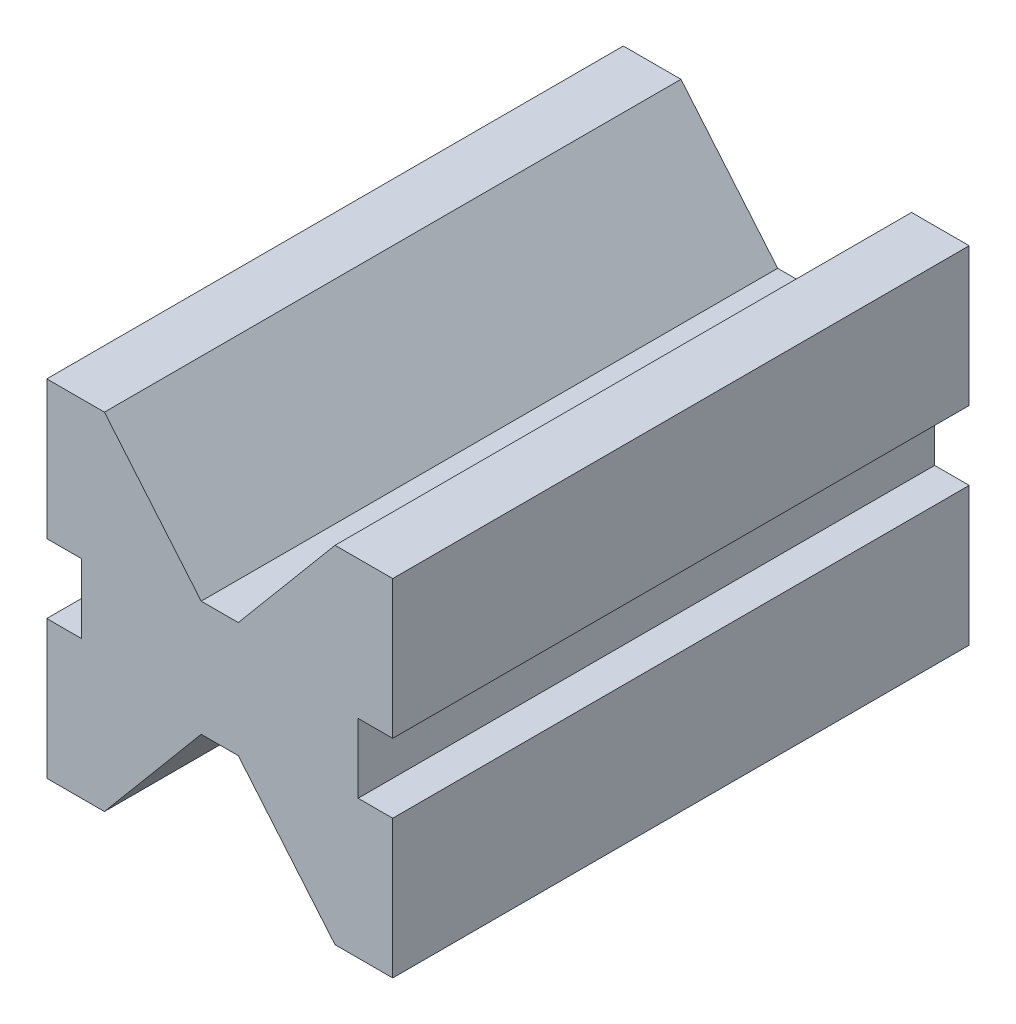
ISO-10303-21;
HEADER;
FILE_DESCRIPTION(('STEP AP214'),'2;1');
FILE_NAME('part.step','',(''),(''),'','','');
FILE_SCHEMA(('AUTOMOTIVE_DESIGN { 1 0 10303 214 1 1 1 1 }'));
ENDSEC;
DATA;
#1=APPLICATION_CONTEXT('core data for automotive mechanical design processes');
#2=APPLICATION_PROTOCOL_DEFINITION('international standard','automotive_design',2000,#1);
#3=PRODUCT_CONTEXT('',#1,'mechanical');
#4=PRODUCT('Part','Part','',(#3));
#5=PRODUCT_RELATED_PRODUCT_CATEGORY('part','',(#4));
#6=PRODUCT_DEFINITION_FORMATION('','',#4);
#7=PRODUCT_DEFINITION_CONTEXT('part definition',#1,'design');
#8=PRODUCT_DEFINITION('design','',#6,#7);
#9=PRODUCT_DEFINITION_SHAPE('','',#8);
#10=(LENGTH_UNIT() NAMED_UNIT(*) SI_UNIT(.MILLI.,.METRE.));
#11=(NAMED_UNIT(*) PLANE_ANGLE_UNIT() SI_UNIT($,.RADIAN.));
#12=(NAMED_UNIT(*) SI_UNIT($,.STERADIAN.) SOLID_ANGLE_UNIT());
#13=UNCERTAINTY_MEASURE_WITH_UNIT(LENGTH_MEASURE(1.E-05),#10,'distance_accuracy_value','');
#14=(GEOMETRIC_REPRESENTATION_CONTEXT(3) GLOBAL_UNCERTAINTY_ASSIGNED_CONTEXT((#13)) GLOBAL_UNIT_ASSIGNED_CONTEXT((#10,
#11,#12)) REPRESENTATION_CONTEXT('',''));
#15=CARTESIAN_POINT('',(0.,0.,0.));
#16=DIRECTION('',(0.,0.,1.));
#17=DIRECTION('',(1.,0.,0.));
#18=AXIS2_PLACEMENT_3D('',#15,#16,#17);
#19=CARTESIAN_POINT('',(3.03563451851378,2.54719980487392,-100.));
#20=DIRECTION('',(-0.766044443118979,-0.642787609686538,0.));
#21=DIRECTION('',(0.642787609686538,-0.766044443118979,0.));
#22=AXIS2_PLACEMENT_3D('',#19,#20,#21);
#23=PLANE('',#22);
#24=DIRECTION('',(0.642787609686538,-0.766044443118979,0.));
#25=VECTOR('',#24,1.);
#26=CARTESIAN_POINT('',(3.03563451851378,2.54719980487392,0.));
#27=LINE('',#26,#25);
#28=CARTESIAN_POINT('',(-20.,30.,0.));
#29=VERTEX_POINT('',#28);
#30=CARTESIAN_POINT('',(-3.21800737645446,10.,0.));
#31=VERTEX_POINT('',#30);
#32=EDGE_CURVE('E209',#29,#31,#27,.T.);
#33=ORIENTED_EDGE('',*,*,#32,.T.);
#34=DIRECTION('',(0.,0.,1.));
#35=VECTOR('',#34,1.);
#36=CARTESIAN_POINT('',(-3.21800737645446,10.,-100.));
#37=LINE('',#36,#35);
#38=CARTESIAN_POINT('',(-3.21800737645446,10.,-100.));
#39=VERTEX_POINT('',#38);
#40=EDGE_CURVE('E11',#39,#31,#37,.T.);
#41=ORIENTED_EDGE('',*,*,#40,.F.);
#42=DIRECTION('',(0.642787609686538,-0.766044443118979,0.));
#43=VECTOR('',#42,1.);
#44=CARTESIAN_POINT('',(3.03563451851378,2.54719980487392,-100.));
#45=LINE('',#44,#43);
#46=CARTESIAN_POINT('',(-20.,30.,-100.));
#47=VERTEX_POINT('',#46);
#48=EDGE_CURVE('E257',#47,#39,#45,.T.);
#49=ORIENTED_EDGE('',*,*,#48,.F.);
#50=DIRECTION('',(0.,0.,1.));
#51=VECTOR('',#50,1.);
#52=CARTESIAN_POINT('',(-20.,30.,-100.));
#53=LINE('',#52,#51);
#54=EDGE_CURVE('E42',#47,#29,#53,.T.);
#55=ORIENTED_EDGE('',*,*,#54,.T.);
#56=EDGE_LOOP('',(#33,#41,#49,#55));
#57=FACE_BOUND('',#56,.T.);
#58=ADVANCED_FACE('F41',(#57),#23,.F.);
#59=CARTESIAN_POINT('',(0.,10.,-100.));
#60=DIRECTION('',(0.,-1.,0.));
#61=DIRECTION('',(1.,0.,0.));
#62=AXIS2_PLACEMENT_3D('',#59,#60,#61);
#63=PLANE('',#62);
#64=DIRECTION('',(1.,0.,0.));
#65=VECTOR('',#64,1.);
#66=CARTESIAN_POINT('',(0.,10.,0.));
#67=LINE('',#66,#65);
#68=CARTESIAN_POINT('',(3.21800737645446,10.,0.));
#69=VERTEX_POINT('',#68);
#70=EDGE_CURVE('E126',#31,#69,#67,.T.);
#71=ORIENTED_EDGE('',*,*,#70,.T.);
#72=DIRECTION('',(0.,0.,1.));
#73=VECTOR('',#72,1.);
#74=CARTESIAN_POINT('',(3.21800737645446,10.,-100.));
#75=LINE('',#74,#73);
#76=CARTESIAN_POINT('',(3.21800737645446,10.,-100.));
#77=VERTEX_POINT('',#76);
#78=EDGE_CURVE('E49',#77,#69,#75,.T.);
#79=ORIENTED_EDGE('',*,*,#78,.F.);
#80=DIRECTION('',(1.,0.,0.));
#81=VECTOR('',#80,1.);
#82=CARTESIAN_POINT('',(0.,10.,-100.));
#83=LINE('',#82,#81);
#84=EDGE_CURVE('E59',#39,#77,#83,.T.);
#85=ORIENTED_EDGE('',*,*,#84,.F.);
#86=ORIENTED_EDGE('',*,*,#40,.T.);
#87=EDGE_LOOP('',(#71,#79,#85,#86));
#88=FACE_BOUND('',#87,.T.);
#89=ADVANCED_FACE('F311',(#88),#63,.F.);
#90=CARTESIAN_POINT('',(-3.03563451851378,2.54719980487392,-100.));
#91=DIRECTION('',(-0.766044443118979,0.642787609686538,0.));
#92=DIRECTION('',(-0.642787609686538,-0.766044443118979,0.));
#93=AXIS2_PLACEMENT_3D('',#90,#91,#92);
#94=PLANE('',#93);
#95=DIRECTION('',(-0.642787609686538,-0.766044443118979,0.));
#96=VECTOR('',#95,1.);
#97=CARTESIAN_POINT('',(-3.03563451851378,2.54719980487392,0.));
#98=LINE('',#97,#96);
#99=CARTESIAN_POINT('',(20.,30.,0.));
#100=VERTEX_POINT('',#99);
#101=EDGE_CURVE('E187',#100,#69,#98,.T.);
#102=ORIENTED_EDGE('',*,*,#101,.F.);
#103=DIRECTION('',(0.,0.,1.));
#104=VECTOR('',#103,1.);
#105=CARTESIAN_POINT('',(20.,30.,-100.));
#106=LINE('',#105,#104);
#107=CARTESIAN_POINT('',(20.,30.,-100.));
#108=VERTEX_POINT('',#107);
#109=EDGE_CURVE('E184',#108,#100,#106,.T.);
#110=ORIENTED_EDGE('',*,*,#109,.F.);
#111=DIRECTION('',(-0.642787609686538,-0.766044443118979,0.));
#112=VECTOR('',#111,1.);
#113=CARTESIAN_POINT('',(-3.03563451851378,2.54719980487392,-100.));
#114=LINE('',#113,#112);
#115=EDGE_CURVE('E190',#108,#77,#114,.T.);
#116=ORIENTED_EDGE('',*,*,#115,.T.);
#117=ORIENTED_EDGE('',*,*,#78,.T.);
#118=EDGE_LOOP('',(#102,#110,#116,#117));
#119=FACE_BOUND('',#118,.T.);
#120=ADVANCED_FACE('F186',(#119),#94,.T.);
#121=CARTESIAN_POINT('',(0.,30.,-100.));
#122=DIRECTION('',(0.,1.,0.));
#123=DIRECTION('',(-1.,0.,0.));
#124=AXIS2_PLACEMENT_3D('',#121,#122,#123);
#125=PLANE('',#124);
#126=DIRECTION('',(-1.,0.,0.));
#127=VECTOR('',#126,1.);
#128=CARTESIAN_POINT('',(0.,30.,0.));
#129=LINE('',#128,#127);
#130=CARTESIAN_POINT('',(30.,30.,0.));
#131=VERTEX_POINT('',#130);
#132=EDGE_CURVE('E260',#131,#100,#129,.T.);
#133=ORIENTED_EDGE('',*,*,#132,.F.);
#134=DIRECTION('',(0.,0.,1.));
#135=VECTOR('',#134,1.);
#136=CARTESIAN_POINT('',(30.,30.,-100.));
#137=LINE('',#136,#135);
#138=CARTESIAN_POINT('',(30.,30.,-100.));
#139=VERTEX_POINT('',#138);
#140=EDGE_CURVE('E195',#139,#131,#137,.T.);
#141=ORIENTED_EDGE('',*,*,#140,.F.);
#142=DIRECTION('',(-1.,0.,0.));
#143=VECTOR('',#142,1.);
#144=CARTESIAN_POINT('',(0.,30.,-100.));
#145=LINE('',#144,#143);
#146=EDGE_CURVE('E200',#139,#108,#145,.T.);
#147=ORIENTED_EDGE('',*,*,#146,.T.);
#148=ORIENTED_EDGE('',*,*,#109,.T.);
#149=EDGE_LOOP('',(#133,#141,#147,#148));
#150=FACE_BOUND('',#149,.T.);
#151=ADVANCED_FACE('F205',(#150),#125,.T.);
#152=CARTESIAN_POINT('',(30.,0.,-100.));
#153=DIRECTION('',(1.,0.,0.));
#154=DIRECTION('',(0.,0.,-1.));
#155=AXIS2_PLACEMENT_3D('',#152,#153,#154);
#156=PLANE('',#155);
#157=DIRECTION('',(0.,1.,0.));
#158=VECTOR('',#157,1.);
#159=CARTESIAN_POINT('',(30.,0.,0.));
#160=LINE('',#159,#158);
#161=CARTESIAN_POINT('',(30.,5.99999999999999,0.));
#162=VERTEX_POINT('',#161);
#163=EDGE_CURVE('E255',#162,#131,#160,.T.);
#164=ORIENTED_EDGE('',*,*,#163,.F.);
#165=DIRECTION('',(0.,0.,1.));
#166=VECTOR('',#165,1.);
#167=CARTESIAN_POINT('',(30.,5.99999999999999,-100.));
#168=LINE('',#167,#166);
#169=CARTESIAN_POINT('',(30.,5.99999999999999,-100.));
#170=VERTEX_POINT('',#169);
#171=EDGE_CURVE('E262',#170,#162,#168,.T.);
#172=ORIENTED_EDGE('',*,*,#171,.F.);
#173=DIRECTION('',(0.,1.,0.));
#174=VECTOR('',#173,1.);
#175=CARTESIAN_POINT('',(30.,0.,-100.));
#176=LINE('',#175,#174);
#177=EDGE_CURVE('E201',#170,#139,#176,.T.);
#178=ORIENTED_EDGE('',*,*,#177,.T.);
#179=ORIENTED_EDGE('',*,*,#140,.T.);
#180=EDGE_LOOP('',(#164,#172,#178,#179));
#181=FACE_BOUND('',#180,.T.);
#182=ADVANCED_FACE('F326',(#181),#156,.T.);
#183=CARTESIAN_POINT('',(0.,5.99999999999999,-100.));
#184=DIRECTION('',(0.,1.,0.));
#185=DIRECTION('',(-1.,0.,0.));
#186=AXIS2_PLACEMENT_3D('',#183,#184,#185);
#187=PLANE('',#186);
#188=DIRECTION('',(-1.,0.,0.));
#189=VECTOR('',#188,1.);
#190=CARTESIAN_POINT('',(0.,5.99999999999999,0.));
#191=LINE('',#190,#189);
#192=CARTESIAN_POINT('',(24.,5.99999999999999,0.));
#193=VERTEX_POINT('',#192);
#194=EDGE_CURVE('E252',#162,#193,#191,.T.);
#195=ORIENTED_EDGE('',*,*,#194,.T.);
#196=DIRECTION('',(0.,0.,1.));
#197=VECTOR('',#196,1.);
#198=CARTESIAN_POINT('',(24.,5.99999999999999,-100.));
#199=LINE('',#198,#197);
#200=CARTESIAN_POINT('',(24.,5.99999999999999,-100.));
#201=VERTEX_POINT('',#200);
#202=EDGE_CURVE('E266',#201,#193,#199,.T.);
#203=ORIENTED_EDGE('',*,*,#202,.F.);
#204=DIRECTION('',(-1.,0.,0.));
#205=VECTOR('',#204,1.);
#206=CARTESIAN_POINT('',(0.,5.99999999999999,-100.));
#207=LINE('',#206,#205);
#208=EDGE_CURVE('E202',#170,#201,#207,.T.);
#209=ORIENTED_EDGE('',*,*,#208,.F.);
#210=ORIENTED_EDGE('',*,*,#171,.T.);
#211=EDGE_LOOP('',(#195,#203,#209,#210));
#212=FACE_BOUND('',#211,.T.);
#213=ADVANCED_FACE('F328',(#212),#187,.F.);
#214=CARTESIAN_POINT('',(24.,0.,-100.));
#215=DIRECTION('',(-1.,0.,0.));
#216=DIRECTION('',(0.,0.,1.));
#217=AXIS2_PLACEMENT_3D('',#214,#215,#216);
#218=PLANE('',#217);
#219=DIRECTION('',(0.,-1.,0.));
#220=VECTOR('',#219,1.);
#221=CARTESIAN_POINT('',(24.,0.,0.));
#222=LINE('',#221,#220);
#223=CARTESIAN_POINT('',(24.,-6.00000000000001,0.));
#224=VERTEX_POINT('',#223);
#225=EDGE_CURVE('E248',#193,#224,#222,.T.);
#226=ORIENTED_EDGE('',*,*,#225,.T.);
#227=DIRECTION('',(0.,0.,1.));
#228=VECTOR('',#227,1.);
#229=CARTESIAN_POINT('',(24.,-6.00000000000001,-100.));
#230=LINE('',#229,#228);
#231=CARTESIAN_POINT('',(24.,-6.00000000000001,-100.));
#232=VERTEX_POINT('',#231);
#233=EDGE_CURVE('E267',#232,#224,#230,.T.);
#234=ORIENTED_EDGE('',*,*,#233,.F.);
#235=DIRECTION('',(0.,-1.,0.));
#236=VECTOR('',#235,1.);
#237=CARTESIAN_POINT('',(24.,0.,-100.));
#238=LINE('',#237,#236);
#239=EDGE_CURVE('E423',#201,#232,#238,.T.);
#240=ORIENTED_EDGE('',*,*,#239,.F.);
#241=ORIENTED_EDGE('',*,*,#202,.T.);
#242=EDGE_LOOP('',(#226,#234,#240,#241));
#243=FACE_BOUND('',#242,.T.);
#244=ADVANCED_FACE('F334',(#243),#218,.F.);
#245=CARTESIAN_POINT('',(0.,-6.00000000000001,-100.));
#246=DIRECTION('',(0.,-1.,0.));
#247=DIRECTION('',(0.,0.,-1.));
#248=AXIS2_PLACEMENT_3D('',#245,#246,#247);
#249=PLANE('',#248);
#250=DIRECTION('',(1.,0.,0.));
#251=VECTOR('',#250,1.);
#252=CARTESIAN_POINT('',(0.,-6.00000000000001,0.));
#253=LINE('',#252,#251);
#254=CARTESIAN_POINT('',(30.,-6.00000000000001,0.));
#255=VERTEX_POINT('',#254);
#256=EDGE_CURVE('E249',#224,#255,#253,.T.);
#257=ORIENTED_EDGE('',*,*,#256,.T.);
#258=DIRECTION('',(0.,0.,1.));
#259=VECTOR('',#258,1.);
#260=CARTESIAN_POINT('',(30.,-6.00000000000001,-100.));
#261=LINE('',#260,#259);
#262=CARTESIAN_POINT('',(30.,-6.00000000000001,-100.));
#263=VERTEX_POINT('',#262);
#264=EDGE_CURVE('E275',#263,#255,#261,.T.);
#265=ORIENTED_EDGE('',*,*,#264,.F.);
#266=DIRECTION('',(1.,0.,0.));
#267=VECTOR('',#266,1.);
#268=CARTESIAN_POINT('',(0.,-6.00000000000001,-100.));
#269=LINE('',#268,#267);
#270=EDGE_CURVE('E420',#232,#263,#269,.T.);
#271=ORIENTED_EDGE('',*,*,#270,.F.);
#272=ORIENTED_EDGE('',*,*,#233,.T.);
#273=EDGE_LOOP('',(#257,#265,#271,#272));
#274=FACE_BOUND('',#273,.T.);
#275=ADVANCED_FACE('F340',(#274),#249,.F.);
#276=CARTESIAN_POINT('',(30.,0.,-100.));
#277=DIRECTION('',(1.,0.,0.));
#278=DIRECTION('',(0.,0.,-1.));
#279=AXIS2_PLACEMENT_3D('',#276,#277,#278);
#280=PLANE('',#279);
#281=DIRECTION('',(0.,1.,0.));
#282=VECTOR('',#281,1.);
#283=CARTESIAN_POINT('',(30.,0.,0.));
#284=LINE('',#283,#282);
#285=CARTESIAN_POINT('',(30.,-30.,0.));
#286=VERTEX_POINT('',#285);
#287=EDGE_CURVE('E243',#286,#255,#284,.T.);
#288=ORIENTED_EDGE('',*,*,#287,.F.);
#289=DIRECTION('',(0.,0.,1.));
#290=VECTOR('',#289,1.);
#291=CARTESIAN_POINT('',(30.,-30.,-100.));
#292=LINE('',#291,#290);
#293=CARTESIAN_POINT('',(30.,-30.,-100.));
#294=VERTEX_POINT('',#293);
#295=EDGE_CURVE('E273',#294,#286,#292,.T.);
#296=ORIENTED_EDGE('',*,*,#295,.F.);
#297=DIRECTION('',(0.,1.,0.));
#298=VECTOR('',#297,1.);
#299=CARTESIAN_POINT('',(30.,0.,-100.));
#300=LINE('',#299,#298);
#301=EDGE_CURVE('E418',#294,#263,#300,.T.);
#302=ORIENTED_EDGE('',*,*,#301,.T.);
#303=ORIENTED_EDGE('',*,*,#264,.T.);
#304=EDGE_LOOP('',(#288,#296,#302,#303));
#305=FACE_BOUND('',#304,.T.);
#306=ADVANCED_FACE('F342',(#305),#280,.T.);
#307=CARTESIAN_POINT('',(0.,-30.,-100.));
#308=DIRECTION('',(0.,-1.,0.));
#309=DIRECTION('',(0.,0.,-1.));
#310=AXIS2_PLACEMENT_3D('',#307,#308,#309);
#311=PLANE('',#310);
#312=DIRECTION('',(1.,0.,0.));
#313=VECTOR('',#312,1.);
#314=CARTESIAN_POINT('',(0.,-30.,0.));
#315=LINE('',#314,#313);
#316=CARTESIAN_POINT('',(20.,-30.,0.));
#317=VERTEX_POINT('',#316);
#318=EDGE_CURVE('E241',#317,#286,#315,.T.);
#319=ORIENTED_EDGE('',*,*,#318,.F.);
#320=DIRECTION('',(0.,0.,1.));
#321=VECTOR('',#320,1.);
#322=CARTESIAN_POINT('',(20.,-30.,-100.));
#323=LINE('',#322,#321);
#324=CARTESIAN_POINT('',(20.,-30.,-100.));
#325=VERTEX_POINT('',#324);
#326=EDGE_CURVE('E277',#325,#317,#323,.T.);
#327=ORIENTED_EDGE('',*,*,#326,.F.);
#328=DIRECTION('',(1.,0.,0.));
#329=VECTOR('',#328,1.);
#330=CARTESIAN_POINT('',(0.,-30.,-100.));
#331=LINE('',#330,#329);
#332=EDGE_CURVE('E415',#325,#294,#331,.T.);
#333=ORIENTED_EDGE('',*,*,#332,.T.);
#334=ORIENTED_EDGE('',*,*,#295,.T.);
#335=EDGE_LOOP('',(#319,#327,#333,#334));
#336=FACE_BOUND('',#335,.T.);
#337=ADVANCED_FACE('F343',(#336),#311,.T.);
#338=CARTESIAN_POINT('',(-3.03563451851378,-2.54719980487392,-100.));
#339=DIRECTION('',(0.766044443118979,0.642787609686538,0.));
#340=DIRECTION('',(-0.642787609686538,0.766044443118979,0.));
#341=AXIS2_PLACEMENT_3D('',#338,#339,#340);
#342=PLANE('',#341);
#343=DIRECTION('',(-0.642787609686538,0.766044443118979,0.));
#344=VECTOR('',#343,1.);
#345=CARTESIAN_POINT('',(-3.03563451851378,-2.54719980487392,0.));
#346=LINE('',#345,#344);
#347=CARTESIAN_POINT('',(3.21800737645446,-10.,0.));
#348=VERTEX_POINT('',#347);
#349=EDGE_CURVE('E239',#317,#348,#346,.T.);
#350=ORIENTED_EDGE('',*,*,#349,.T.);
#351=DIRECTION('',(0.,0.,1.));
#352=VECTOR('',#351,1.);
#353=CARTESIAN_POINT('',(3.21800737645446,-10.,-100.));
#354=LINE('',#353,#352);
#355=CARTESIAN_POINT('',(3.21800737645446,-10.,-100.));
#356=VERTEX_POINT('',#355);
#357=EDGE_CURVE('E279',#356,#348,#354,.T.);
#358=ORIENTED_EDGE('',*,*,#357,.F.);
#359=DIRECTION('',(-0.642787609686538,0.766044443118979,0.));
#360=VECTOR('',#359,1.);
#361=CARTESIAN_POINT('',(-3.03563451851378,-2.54719980487392,-100.));
#362=LINE('',#361,#360);
#363=EDGE_CURVE('E412',#325,#356,#362,.T.);
#364=ORIENTED_EDGE('',*,*,#363,.F.);
#365=ORIENTED_EDGE('',*,*,#326,.T.);
#366=EDGE_LOOP('',(#350,#358,#364,#365));
#367=FACE_BOUND('',#366,.T.);
#368=ADVANCED_FACE('F349',(#367),#342,.F.);
#369=CARTESIAN_POINT('',(0.,-10.,-100.));
#370=DIRECTION('',(0.,1.,0.));
#371=DIRECTION('',(-1.,0.,0.));
#372=AXIS2_PLACEMENT_3D('',#369,#370,#371);
#373=PLANE('',#372);
#374=DIRECTION('',(-1.,0.,0.));
#375=VECTOR('',#374,1.);
#376=CARTESIAN_POINT('',(0.,-10.,0.));
#377=LINE('',#376,#375);
#378=CARTESIAN_POINT('',(-3.21800737645446,-10.,0.));
#379=VERTEX_POINT('',#378);
#380=EDGE_CURVE('E237',#348,#379,#377,.T.);
#381=ORIENTED_EDGE('',*,*,#380,.T.);
#382=DIRECTION('',(0.,0.,1.));
#383=VECTOR('',#382,1.);
#384=CARTESIAN_POINT('',(-3.21800737645446,-10.,-100.));
#385=LINE('',#384,#383);
#386=CARTESIAN_POINT('',(-3.21800737645446,-10.,-100.));
#387=VERTEX_POINT('',#386);
#388=EDGE_CURVE('E281',#387,#379,#385,.T.);
#389=ORIENTED_EDGE('',*,*,#388,.F.);
#390=DIRECTION('',(-1.,0.,0.));
#391=VECTOR('',#390,1.);
#392=CARTESIAN_POINT('',(0.,-10.,-100.));
#393=LINE('',#392,#391);
#394=EDGE_CURVE('E408',#356,#387,#393,.T.);
#395=ORIENTED_EDGE('',*,*,#394,.F.);
#396=ORIENTED_EDGE('',*,*,#357,.T.);
#397=EDGE_LOOP('',(#381,#389,#395,#396));
#398=FACE_BOUND('',#397,.T.);
#399=ADVANCED_FACE('F352',(#398),#373,.F.);
#400=CARTESIAN_POINT('',(3.03563451851378,-2.54719980487392,-100.));
#401=DIRECTION('',(0.766044443118979,-0.642787609686538,0.));
#402=DIRECTION('',(0.642787609686538,0.766044443118979,0.));
#403=AXIS2_PLACEMENT_3D('',#400,#401,#402);
#404=PLANE('',#403);
#405=DIRECTION('',(0.642787609686538,0.766044443118979,0.));
#406=VECTOR('',#405,1.);
#407=CARTESIAN_POINT('',(3.03563451851378,-2.54719980487392,0.));
#408=LINE('',#407,#406);
#409=CARTESIAN_POINT('',(-20.,-30.,0.));
#410=VERTEX_POINT('',#409);
#411=EDGE_CURVE('E235',#410,#379,#408,.T.);
#412=ORIENTED_EDGE('',*,*,#411,.F.);
#413=DIRECTION('',(0.,0.,1.));
#414=VECTOR('',#413,1.);
#415=CARTESIAN_POINT('',(-20.,-30.,-100.));
#416=LINE('',#415,#414);
#417=CARTESIAN_POINT('',(-20.,-30.,-100.));
#418=VERTEX_POINT('',#417);
#419=EDGE_CURVE('E282',#418,#410,#416,.T.);
#420=ORIENTED_EDGE('',*,*,#419,.F.);
#421=DIRECTION('',(0.642787609686538,0.766044443118979,0.));
#422=VECTOR('',#421,1.);
#423=CARTESIAN_POINT('',(3.03563451851378,-2.54719980487392,-100.));
#424=LINE('',#423,#422);
#425=EDGE_CURVE('E406',#418,#387,#424,.T.);
#426=ORIENTED_EDGE('',*,*,#425,.T.);
#427=ORIENTED_EDGE('',*,*,#388,.T.);
#428=EDGE_LOOP('',(#412,#420,#426,#427));
#429=FACE_BOUND('',#428,.T.);
#430=ADVANCED_FACE('F359',(#429),#404,.T.);
#431=CARTESIAN_POINT('',(0.,-30.,-100.));
#432=DIRECTION('',(0.,-1.,0.));
#433=DIRECTION('',(0.,0.,-1.));
#434=AXIS2_PLACEMENT_3D('',#431,#432,#433);
#435=PLANE('',#434);
#436=DIRECTION('',(1.,0.,0.));
#437=VECTOR('',#436,1.);
#438=CARTESIAN_POINT('',(0.,-30.,0.));
#439=LINE('',#438,#437);
#440=CARTESIAN_POINT('',(-30.,-30.,0.));
#441=VERTEX_POINT('',#440);
#442=EDGE_CURVE('E229',#441,#410,#439,.T.);
#443=ORIENTED_EDGE('',*,*,#442,.F.);
#444=DIRECTION('',(0.,0.,1.));
#445=VECTOR('',#444,1.);
#446=CARTESIAN_POINT('',(-30.,-30.,-100.));
#447=LINE('',#446,#445);
#448=CARTESIAN_POINT('',(-30.,-30.,-100.));
#449=VERTEX_POINT('',#448);
#450=EDGE_CURVE('E284',#449,#441,#447,.T.);
#451=ORIENTED_EDGE('',*,*,#450,.F.);
#452=DIRECTION('',(1.,0.,0.));
#453=VECTOR('',#452,1.);
#454=CARTESIAN_POINT('',(0.,-30.,-100.));
#455=LINE('',#454,#453);
#456=EDGE_CURVE('E401',#449,#418,#455,.T.);
#457=ORIENTED_EDGE('',*,*,#456,.T.);
#458=ORIENTED_EDGE('',*,*,#419,.T.);
#459=EDGE_LOOP('',(#443,#451,#457,#458));
#460=FACE_BOUND('',#459,.T.);
#461=ADVANCED_FACE('F363',(#460),#435,.T.);
#462=CARTESIAN_POINT('',(-30.,0.,-100.));
#463=DIRECTION('',(1.,0.,0.));
#464=DIRECTION('',(0.,1.,0.));
#465=AXIS2_PLACEMENT_3D('',#462,#463,#464);
#466=PLANE('',#465);
#467=DIRECTION('',(0.,1.,0.));
#468=VECTOR('',#467,1.);
#469=CARTESIAN_POINT('',(-30.,0.,0.));
#470=LINE('',#469,#468);
#471=CARTESIAN_POINT('',(-30.,-6.00000000000001,0.));
#472=VERTEX_POINT('',#471);
#473=EDGE_CURVE('E227',#441,#472,#470,.T.);
#474=ORIENTED_EDGE('',*,*,#473,.T.);
#475=DIRECTION('',(0.,0.,1.));
#476=VECTOR('',#475,1.);
#477=CARTESIAN_POINT('',(-30.,-6.00000000000001,-100.));
#478=LINE('',#477,#476);
#479=CARTESIAN_POINT('',(-30.,-6.00000000000001,-100.));
#480=VERTEX_POINT('',#479);
#481=EDGE_CURVE('E289',#480,#472,#478,.T.);
#482=ORIENTED_EDGE('',*,*,#481,.F.);
#483=DIRECTION('',(0.,1.,0.));
#484=VECTOR('',#483,1.);
#485=CARTESIAN_POINT('',(-30.,0.,-100.));
#486=LINE('',#485,#484);
#487=EDGE_CURVE('E402',#449,#480,#486,.T.);
#488=ORIENTED_EDGE('',*,*,#487,.F.);
#489=ORIENTED_EDGE('',*,*,#450,.T.);
#490=EDGE_LOOP('',(#474,#482,#488,#489));
#491=FACE_BOUND('',#490,.T.);
#492=ADVANCED_FACE('F364',(#491),#466,.F.);
#493=CARTESIAN_POINT('',(0.,-6.00000000000001,-100.));
#494=DIRECTION('',(0.,-1.,0.));
#495=DIRECTION('',(0.,0.,-1.));
#496=AXIS2_PLACEMENT_3D('',#493,#494,#495);
#497=PLANE('',#496);
#498=DIRECTION('',(1.,0.,0.));
#499=VECTOR('',#498,1.);
#500=CARTESIAN_POINT('',(0.,-6.00000000000001,0.));
#501=LINE('',#500,#499);
#502=CARTESIAN_POINT('',(-24.,-6.00000000000001,0.));
#503=VERTEX_POINT('',#502);
#504=EDGE_CURVE('E223',#472,#503,#501,.T.);
#505=ORIENTED_EDGE('',*,*,#504,.T.);
#506=DIRECTION('',(0.,0.,1.));
#507=VECTOR('',#506,1.);
#508=CARTESIAN_POINT('',(-24.,-6.00000000000001,-100.));
#509=LINE('',#508,#507);
#510=CARTESIAN_POINT('',(-24.,-6.00000000000001,-100.));
#511=VERTEX_POINT('',#510);
#512=EDGE_CURVE('E288',#511,#503,#509,.T.);
#513=ORIENTED_EDGE('',*,*,#512,.F.);
#514=DIRECTION('',(1.,0.,0.));
#515=VECTOR('',#514,1.);
#516=CARTESIAN_POINT('',(0.,-6.00000000000001,-100.));
#517=LINE('',#516,#515);
#518=EDGE_CURVE('E396',#480,#511,#517,.T.);
#519=ORIENTED_EDGE('',*,*,#518,.F.);
#520=ORIENTED_EDGE('',*,*,#481,.T.);
#521=EDGE_LOOP('',(#505,#513,#519,#520));
#522=FACE_BOUND('',#521,.T.);
#523=ADVANCED_FACE('F369',(#522),#497,.F.);
#524=CARTESIAN_POINT('',(-24.,0.,-100.));
#525=DIRECTION('',(-1.,0.,0.));
#526=DIRECTION('',(0.,0.,1.));
#527=AXIS2_PLACEMENT_3D('',#524,#525,#526);
#528=PLANE('',#527);
#529=DIRECTION('',(0.,-1.,0.));
#530=VECTOR('',#529,1.);
#531=CARTESIAN_POINT('',(-24.,0.,0.));
#532=LINE('',#531,#530);
#533=CARTESIAN_POINT('',(-24.,5.99999999999999,0.));
#534=VERTEX_POINT('',#533);
#535=EDGE_CURVE('E225',#534,#503,#532,.T.);
#536=ORIENTED_EDGE('',*,*,#535,.F.);
#537=DIRECTION('',(0.,0.,1.));
#538=VECTOR('',#537,1.);
#539=CARTESIAN_POINT('',(-24.,5.99999999999999,-100.));
#540=LINE('',#539,#538);
#541=CARTESIAN_POINT('',(-24.,5.99999999999999,-100.));
#542=VERTEX_POINT('',#541);
#543=EDGE_CURVE('E295',#542,#534,#540,.T.);
#544=ORIENTED_EDGE('',*,*,#543,.F.);
#545=DIRECTION('',(0.,-1.,0.));
#546=VECTOR('',#545,1.);
#547=CARTESIAN_POINT('',(-24.,0.,-100.));
#548=LINE('',#547,#546);
#549=EDGE_CURVE('E395',#542,#511,#548,.T.);
#550=ORIENTED_EDGE('',*,*,#549,.T.);
#551=ORIENTED_EDGE('',*,*,#512,.T.);
#552=EDGE_LOOP('',(#536,#544,#550,#551));
#553=FACE_BOUND('',#552,.T.);
#554=ADVANCED_FACE('F373',(#553),#528,.T.);
#555=CARTESIAN_POINT('',(0.,5.99999999999999,-100.));
#556=DIRECTION('',(0.,-1.,0.));
#557=DIRECTION('',(0.,0.,-1.));
#558=AXIS2_PLACEMENT_3D('',#555,#556,#557);
#559=PLANE('',#558);
#560=DIRECTION('',(1.,0.,0.));
#561=VECTOR('',#560,1.);
#562=CARTESIAN_POINT('',(0.,5.99999999999999,0.));
#563=LINE('',#562,#561);
#564=CARTESIAN_POINT('',(-30.,5.99999999999999,0.));
#565=VERTEX_POINT('',#564);
#566=EDGE_CURVE('E218',#565,#534,#563,.T.);
#567=ORIENTED_EDGE('',*,*,#566,.F.);
#568=DIRECTION('',(0.,0.,1.));
#569=VECTOR('',#568,1.);
#570=CARTESIAN_POINT('',(-30.,5.99999999999999,-100.));
#571=LINE('',#570,#569);
#572=CARTESIAN_POINT('',(-30.,5.99999999999999,-100.));
#573=VERTEX_POINT('',#572);
#574=EDGE_CURVE('E294',#573,#565,#571,.T.);
#575=ORIENTED_EDGE('',*,*,#574,.F.);
#576=DIRECTION('',(1.,0.,0.));
#577=VECTOR('',#576,1.);
#578=CARTESIAN_POINT('',(0.,5.99999999999999,-100.));
#579=LINE('',#578,#577);
#580=EDGE_CURVE('E386',#573,#542,#579,.T.);
#581=ORIENTED_EDGE('',*,*,#580,.T.);
#582=ORIENTED_EDGE('',*,*,#543,.T.);
#583=EDGE_LOOP('',(#567,#575,#581,#582));
#584=FACE_BOUND('',#583,.T.);
#585=ADVANCED_FACE('F310',(#584),#559,.T.);
#586=CARTESIAN_POINT('',(-30.,0.,-100.));
#587=DIRECTION('',(-1.,0.,0.));
#588=DIRECTION('',(0.,0.,1.));
#589=AXIS2_PLACEMENT_3D('',#586,#587,#588);
#590=PLANE('',#589);
#591=DIRECTION('',(0.,-1.,0.));
#592=VECTOR('',#591,1.);
#593=CARTESIAN_POINT('',(-30.,0.,0.));
#594=LINE('',#593,#592);
#595=CARTESIAN_POINT('',(-30.,30.,0.));
#596=VERTEX_POINT('',#595);
#597=EDGE_CURVE('E216',#596,#565,#594,.T.);
#598=ORIENTED_EDGE('',*,*,#597,.F.);
#599=DIRECTION('',(0.,0.,1.));
#600=VECTOR('',#599,1.);
#601=CARTESIAN_POINT('',(-30.,30.,-100.));
#602=LINE('',#601,#600);
#603=CARTESIAN_POINT('',(-30.,30.,-100.));
#604=VERTEX_POINT('',#603);
#605=EDGE_CURVE('E293',#604,#596,#602,.T.);
#606=ORIENTED_EDGE('',*,*,#605,.F.);
#607=DIRECTION('',(0.,-1.,0.));
#608=VECTOR('',#607,1.);
#609=CARTESIAN_POINT('',(-30.,0.,-100.));
#610=LINE('',#609,#608);
#611=EDGE_CURVE('E389',#604,#573,#610,.T.);
#612=ORIENTED_EDGE('',*,*,#611,.T.);
#613=ORIENTED_EDGE('',*,*,#574,.T.);
#614=EDGE_LOOP('',(#598,#606,#612,#613));
#615=FACE_BOUND('',#614,.T.);
#616=ADVANCED_FACE('F305',(#615),#590,.T.);
#617=CARTESIAN_POINT('',(0.,30.,-100.));
#618=DIRECTION('',(0.,1.,0.));
#619=DIRECTION('',(-1.,0.,0.));
#620=AXIS2_PLACEMENT_3D('',#617,#618,#619);
#621=PLANE('',#620);
#622=DIRECTION('',(-1.,0.,0.));
#623=VECTOR('',#622,1.);
#624=CARTESIAN_POINT('',(0.,30.,0.));
#625=LINE('',#624,#623);
#626=EDGE_CURVE('E213',#29,#596,#625,.T.);
#627=ORIENTED_EDGE('',*,*,#626,.F.);
#628=ORIENTED_EDGE('',*,*,#54,.F.);
#629=DIRECTION('',(-1.,0.,0.));
#630=VECTOR('',#629,1.);
#631=CARTESIAN_POINT('',(0.,30.,-100.));
#632=LINE('',#631,#630);
#633=EDGE_CURVE('E388',#47,#604,#632,.T.);
#634=ORIENTED_EDGE('',*,*,#633,.T.);
#635=ORIENTED_EDGE('',*,*,#605,.T.);
#636=EDGE_LOOP('',(#627,#628,#634,#635));
#637=FACE_BOUND('',#636,.T.);
#638=ADVANCED_FACE('F302',(#637),#621,.T.);
#639=CARTESIAN_POINT('',(0.,0.,-100.));
#640=DIRECTION('',(0.,0.,1.));
#641=DIRECTION('',(1.,0.,0.));
#642=AXIS2_PLACEMENT_3D('',#639,#640,#641);
#643=PLANE('',#642);
#644=ORIENTED_EDGE('',*,*,#48,.T.);
#645=ORIENTED_EDGE('',*,*,#84,.T.);
#646=ORIENTED_EDGE('',*,*,#115,.F.);
#647=ORIENTED_EDGE('',*,*,#146,.F.);
#648=ORIENTED_EDGE('',*,*,#177,.F.);
#649=ORIENTED_EDGE('',*,*,#208,.T.);
#650=ORIENTED_EDGE('',*,*,#239,.T.);
#651=ORIENTED_EDGE('',*,*,#270,.T.);
#652=ORIENTED_EDGE('',*,*,#301,.F.);
#653=ORIENTED_EDGE('',*,*,#332,.F.);
#654=ORIENTED_EDGE('',*,*,#363,.T.);
#655=ORIENTED_EDGE('',*,*,#394,.T.);
#656=ORIENTED_EDGE('',*,*,#425,.F.);
#657=ORIENTED_EDGE('',*,*,#456,.F.);
#658=ORIENTED_EDGE('',*,*,#487,.T.);
#659=ORIENTED_EDGE('',*,*,#518,.T.);
#660=ORIENTED_EDGE('',*,*,#549,.F.);
#661=ORIENTED_EDGE('',*,*,#580,.F.);
#662=ORIENTED_EDGE('',*,*,#611,.F.);
#663=ORIENTED_EDGE('',*,*,#633,.F.);
#664=EDGE_LOOP('',(#644,#645,#646,#647,#648,#649,#650,#651,#652,#653,#654,#655,#656,#657,#658,
#659,#660,#661,#662,#663));
#665=FACE_BOUND('',#664,.T.);
#666=ADVANCED_FACE('F197',(#665),#643,.F.);
#667=CARTESIAN_POINT('',(0.,0.,0.));
#668=DIRECTION('',(0.,0.,1.));
#669=DIRECTION('',(1.,0.,0.));
#670=AXIS2_PLACEMENT_3D('',#667,#668,#669);
#671=PLANE('',#670);
#672=ORIENTED_EDGE('',*,*,#32,.F.);
#673=ORIENTED_EDGE('',*,*,#626,.T.);
#674=ORIENTED_EDGE('',*,*,#597,.T.);
#675=ORIENTED_EDGE('',*,*,#566,.T.);
#676=ORIENTED_EDGE('',*,*,#535,.T.);
#677=ORIENTED_EDGE('',*,*,#504,.F.);
#678=ORIENTED_EDGE('',*,*,#473,.F.);
#679=ORIENTED_EDGE('',*,*,#442,.T.);
#680=ORIENTED_EDGE('',*,*,#411,.T.);
#681=ORIENTED_EDGE('',*,*,#380,.F.);
#682=ORIENTED_EDGE('',*,*,#349,.F.);
#683=ORIENTED_EDGE('',*,*,#318,.T.);
#684=ORIENTED_EDGE('',*,*,#287,.T.);
#685=ORIENTED_EDGE('',*,*,#256,.F.);
#686=ORIENTED_EDGE('',*,*,#225,.F.);
#687=ORIENTED_EDGE('',*,*,#194,.F.);
#688=ORIENTED_EDGE('',*,*,#163,.T.);
#689=ORIENTED_EDGE('',*,*,#132,.T.);
#690=ORIENTED_EDGE('',*,*,#101,.T.);
#691=ORIENTED_EDGE('',*,*,#70,.F.);
#692=EDGE_LOOP('',(#672,#673,#674,#675,#676,#677,#678,#679,#680,#681,#682,#683,#684,#685,#686,
#687,#688,#689,#690,#691));
#693=FACE_BOUND('',#692,.T.);
#694=ADVANCED_FACE('F299',(#693),#671,.T.);
#695=CLOSED_SHELL('',(#58,#89,#120,#151,#182,#213,#244,#275,#306,#337,#368,#399,#430,#461,#492,
#523,#554,#585,#616,#638,#666,#694));
#696=MANIFOLD_SOLID_BREP('B2',#695);
#697=ADVANCED_BREP_SHAPE_REPRESENTATION('',(#18,#696),#14);
#698=SHAPE_DEFINITION_REPRESENTATION(#9,#697);
ENDSEC;
END-ISO-10303-21;
